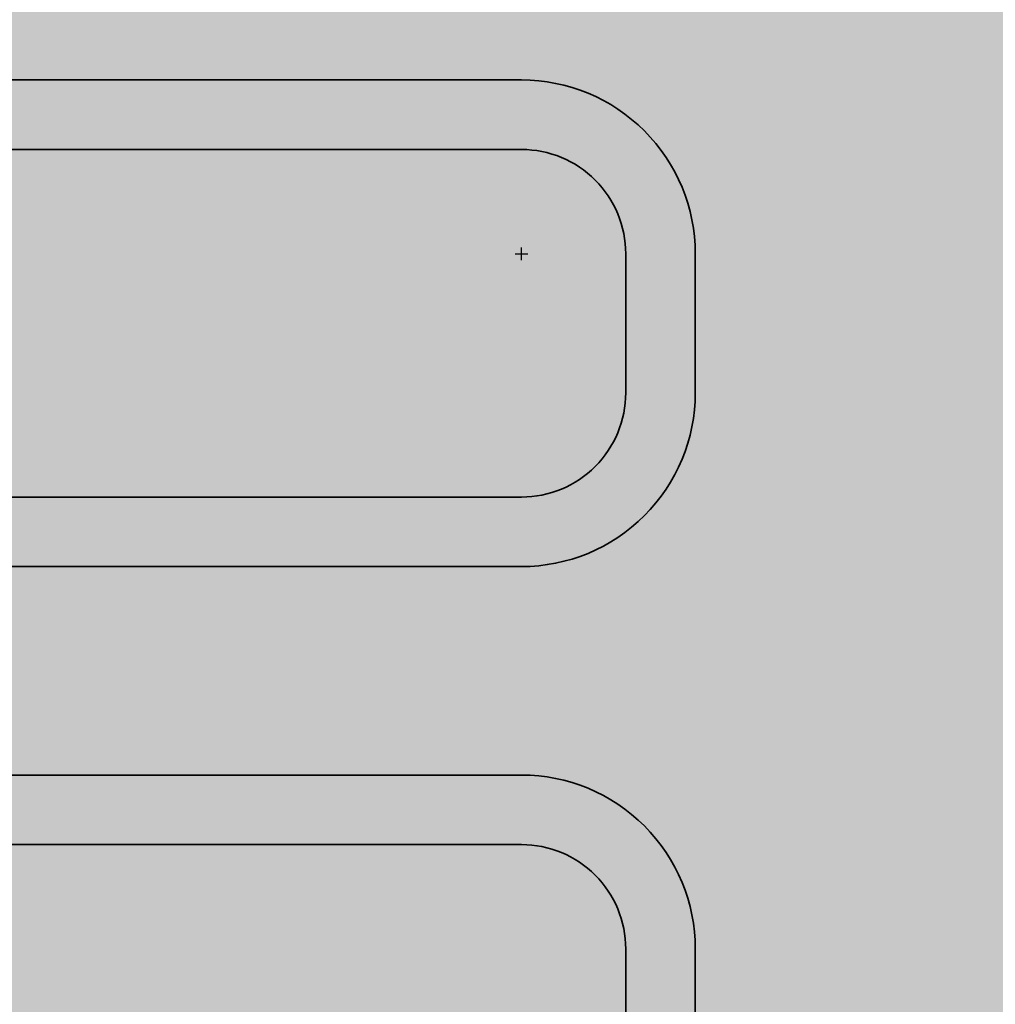
# Model space of a CAD drawing. Units: millimetres. Extents: x -22994 to 29398, y -19990 to 20176.
# Tile 49 of 135: x 169.59 to 183.63, y 110.33 to 124.5. Entities that reach past the tile are written whole.
import ezdxf

# ---------------------------------------------------------------- set-up
doc = ezdxf.new("R2010")
doc.units = ezdxf.units.MM
doc.header["$MEASUREMENT"] = 0
for name, color, linetype, lineweight in [('M-DIMS', 2, 'Continuous', 18), ('M-EQPM-PATT', 7, 'Continuous', 18), ('M-PIPE', 7, 'Continuous', 35)]:
    doc.layers.add(name, color=color, linetype=linetype, lineweight=lineweight)
doc.styles.get("Standard").update_dxf_attribs({"font": 'arial.ttf'})
doc.dimstyles.get("Standard").update_dxf_attribs({"dimtxt": 0.18, "dimasz": 10000, "dimexe": 0.18, "dimexo": 0.0625, "dimgap": 0.09, "dimtad": 0, "dimtih": 1, "dimtoh": 1, "dimdec": 0, "dimzin": 0, "dimdsep": 46, "dimtxsty": 'Standard', "dimcen": 0.09, "dimadec": 0, "dimazin": 0, "dimtfac": 1, "dimtdec": 0, "dimtofl": 0, "dimtmove": 0, "dimatfit": 3, "dimfxl": 1, "dimtolj": 1, "dimtzin": 0, "dimlwd": 30, "dimarcsym": 0})

# ---------------------------------------------------------------- blocks, each defined once
blk = doc.blocks.new('*D2')
at = {"layer": 'Defpoints', "color": 0, "transparency": 16777216}
for p in [(6.677, 10.271), (290.852, 10.271), (290.852, -5.079)]:
    blk.add_point(p, dxfattribs=at)
at = {"layer": 'M-DIMS', "color": 0, "lineweight": -2, "transparency": 16777216}
for p, q in [((6.677, 10.209), (6.677, -5.259)), ((290.852, 10.209), (290.852, -5.259))]:
    blk.add_line(p, q, dxfattribs=at)
at = {"layer": 'M-DIMS', "color": 0, "lineweight": 30, "transparency": 16777216}
for p, q in [((-9993.323, -5.079), (-19993.323, -5.079)), ((10290.852, -5.079), (20290.852, -5.079))]:
    blk.add_line(p, q, dxfattribs=at)
at = {"layer": 'M-DIMS', "color": 0, "transparency": 16777216}
for points in [[(-9993.323, 1661.588), (-9993.323, -1671.745), (6.677, -5.079)], [(10290.852, 1661.588), (10290.852, -1671.745), (290.852, -5.079)]]:
    blk.add_solid(points, dxfattribs=at)
at = {"layer": 'M-DIMS', "color": 0, "transparency": 16777216, "insert": (148.765, -5.079), "char_height": 0.18, "attachment_point": 5}
blk.add_mtext('\\A1;284.2', dxfattribs=at)
blk = doc.blocks.new('*D3')
at = {"layer": 'Defpoints', "color": 0, "transparency": 16777216}
for p in [(110.265, 204.165), (110.265, 176.366), (95.833, 127.967)]:
    blk.add_point(p, dxfattribs=at)
at = {"layer": 'M-DIMS', "color": 0, "lineweight": -2, "transparency": 16777216}
for p, q in [((95.833, 128.03), (95.833, 204.345)), ((110.265, 176.429), (110.265, 204.345))]:
    blk.add_line(p, q, dxfattribs=at)
at = {"layer": 'M-DIMS', "color": 0, "lineweight": 30, "transparency": 16777216}
for p, q in [((-9904.167, 204.165), (-19904.167, 204.165)), ((10110.265, 204.165), (20110.265, 204.165))]:
    blk.add_line(p, q, dxfattribs=at)
at = {"layer": 'M-DIMS', "color": 0, "transparency": 16777216}
for points in [[(-9904.167, 1870.832), (-9904.167, -1462.501), (95.833, 204.165)], [(10110.265, 1870.832), (10110.265, -1462.501), (110.265, 204.165)]]:
    blk.add_solid(points, dxfattribs=at)
at = {"layer": 'M-DIMS', "color": 0, "transparency": 16777216, "insert": (103.049, 204.165), "char_height": 0.18, "attachment_point": 5}
blk.add_mtext('\\A1;14.432', dxfattribs=at)
blk = doc.blocks.new('*D4')
at = {"layer": 'Defpoints', "color": 0, "transparency": 16777216}
for p in [(116.265, 204.165), (110.265, 176.366), (116.265, 176.366)]:
    blk.add_point(p, dxfattribs=at)
at = {"layer": 'M-DIMS', "color": 0, "lineweight": -2, "transparency": 16777216}
for p, q in [((110.265, 176.429), (110.265, 204.345)), ((116.265, 176.429), (116.265, 204.345))]:
    blk.add_line(p, q, dxfattribs=at)
at = {"layer": 'M-DIMS', "color": 0, "lineweight": 30, "transparency": 16777216}
for p, q in [((-9889.735, 204.165), (-19889.735, 204.165)), ((10116.265, 204.165), (20116.265, 204.165))]:
    blk.add_line(p, q, dxfattribs=at)
at = {"layer": 'M-DIMS', "color": 0, "transparency": 16777216}
for points in [[(-9889.735, 1870.832), (-9889.735, -1462.501), (110.265, 204.165)], [(10116.265, 1870.832), (10116.265, -1462.501), (116.265, 204.165)]]:
    blk.add_solid(points, dxfattribs=at)
at = {"layer": 'M-DIMS', "color": 0, "transparency": 16777216, "insert": (113.265, 204.165), "char_height": 0.18, "attachment_point": 5}
blk.add_mtext('\\A1;6', dxfattribs=at)
blk = doc.blocks.new('*D5')
at = {"layer": 'Defpoints', "color": 0, "transparency": 16777216}
for p in [(181.265, 204.165), (116.265, 176.366), (181.265, 176.366)]:
    blk.add_point(p, dxfattribs=at)
at = {"layer": 'M-DIMS', "color": 0, "lineweight": -2, "transparency": 16777216}
for p, q in [((116.265, 176.429), (116.265, 204.345)), ((181.265, 176.429), (181.265, 204.345))]:
    blk.add_line(p, q, dxfattribs=at)
at = {"layer": 'M-DIMS', "color": 0, "lineweight": 30, "transparency": 16777216}
for p, q in [((-9883.735, 204.165), (-19883.735, 204.165)), ((10181.265, 204.165), (20181.265, 204.165))]:
    blk.add_line(p, q, dxfattribs=at)
at = {"layer": 'M-DIMS', "color": 0, "transparency": 16777216}
for points in [[(-9883.735, 1870.832), (-9883.735, -1462.501), (116.265, 204.165)], [(10181.265, 1870.832), (10181.265, -1462.501), (181.265, 204.165)]]:
    blk.add_solid(points, dxfattribs=at)
at = {"layer": 'M-DIMS', "color": 0, "transparency": 16777216, "insert": (148.765, 204.165), "char_height": 0.18, "attachment_point": 5}
blk.add_mtext('\\A1;65', dxfattribs=at)
blk = doc.blocks.new('*D6')
at = {"layer": 'Defpoints', "color": 0, "transparency": 16777216}
for p in [(187.265, 204.165), (181.265, 176.366), (187.265, 176.366)]:
    blk.add_point(p, dxfattribs=at)
at = {"layer": 'M-DIMS', "color": 0, "lineweight": -2, "transparency": 16777216}
for p, q in [((181.265, 176.429), (181.265, 204.345)), ((187.265, 176.429), (187.265, 204.345))]:
    blk.add_line(p, q, dxfattribs=at)
at = {"layer": 'M-DIMS', "color": 0, "lineweight": 30, "transparency": 16777216}
for p, q in [((-9818.735, 204.165), (-19818.735, 204.165)), ((10187.265, 204.165), (20187.265, 204.165))]:
    blk.add_line(p, q, dxfattribs=at)
at = {"layer": 'M-DIMS', "color": 0, "transparency": 16777216}
for points in [[(-9818.735, 1870.832), (-9818.735, -1462.501), (181.265, 204.165)], [(10187.265, 1870.832), (10187.265, -1462.501), (187.265, 204.165)]]:
    blk.add_solid(points, dxfattribs=at)
at = {"layer": 'M-DIMS', "color": 0, "transparency": 16777216, "insert": (184.265, 204.165), "char_height": 0.18, "attachment_point": 5}
blk.add_mtext('\\A1;6', dxfattribs=at)
blk = doc.blocks.new('*D7')
at = {"layer": 'Defpoints', "color": 0, "transparency": 16777216}
for p in [(201.697, 204.165), (187.265, 176.366), (201.697, 127.967)]:
    blk.add_point(p, dxfattribs=at)
at = {"layer": 'M-DIMS', "color": 0, "lineweight": -2, "transparency": 16777216}
for p, q in [((187.265, 176.429), (187.265, 204.345)), ((201.697, 128.03), (201.697, 204.345))]:
    blk.add_line(p, q, dxfattribs=at)
at = {"layer": 'M-DIMS', "color": 0, "lineweight": 30, "transparency": 16777216}
for p, q in [((-9812.735, 204.165), (-19812.735, 204.165)), ((10201.697, 204.165), (20201.697, 204.165))]:
    blk.add_line(p, q, dxfattribs=at)
at = {"layer": 'M-DIMS', "color": 0, "transparency": 16777216}
for points in [[(-9812.735, 1870.832), (-9812.735, -1462.501), (187.265, 204.165)], [(10201.697, 1870.832), (10201.697, -1462.501), (201.697, 204.165)]]:
    blk.add_solid(points, dxfattribs=at)
at = {"layer": 'M-DIMS', "color": 0, "transparency": 16777216, "insert": (194.481, 204.165), "char_height": 0.18, "attachment_point": 5}
blk.add_mtext('\\A1;14.432', dxfattribs=at)
blk = doc.blocks.new('*D8')
at = {"layer": 'Defpoints', "color": 0, "transparency": 16777216}
for p in [(227.648, 204.165), (227.648, 146.73), (201.697, 127.967)]:
    blk.add_point(p, dxfattribs=at)
at = {"layer": 'M-DIMS', "color": 0, "lineweight": -2, "transparency": 16777216}
for p, q in [((201.697, 128.03), (201.697, 204.345)), ((227.648, 146.792), (227.648, 204.345))]:
    blk.add_line(p, q, dxfattribs=at)
at = {"layer": 'M-DIMS', "color": 0, "lineweight": 30, "transparency": 16777216}
for p, q in [((-9798.303, 204.165), (-19798.303, 204.165)), ((10227.648, 204.165), (20227.648, 204.165))]:
    blk.add_line(p, q, dxfattribs=at)
at = {"layer": 'M-DIMS', "color": 0, "transparency": 16777216}
for points in [[(-9798.303, 1870.832), (-9798.303, -1462.501), (201.697, 204.165)], [(10227.648, 1870.832), (10227.648, -1462.501), (227.648, 204.165)]]:
    blk.add_solid(points, dxfattribs=at)
at = {"layer": 'M-DIMS', "color": 0, "transparency": 16777216, "insert": (214.673, 204.165), "char_height": 0.18, "attachment_point": 5}
blk.add_mtext('\\A1;25.95', dxfattribs=at)
blk = doc.blocks.new('*D9')
at = {"layer": 'Defpoints', "color": 0, "transparency": 16777216}
for p in [(187.265, 176.366), (306.202, 176.366), (290.852, 10.271)]:
    blk.add_point(p, dxfattribs=at)
at = {"layer": 'M-DIMS', "color": 0, "lineweight": 30, "transparency": 16777216}
for p, q in [((306.202, 10176.366), (306.202, 20176.366)), ((306.202, -9989.729), (306.202, -19989.729))]:
    blk.add_line(p, q, dxfattribs=at)
at = {"layer": 'M-DIMS', "color": 0, "lineweight": -2, "transparency": 16777216}
for p, q in [((187.327, 176.366), (306.382, 176.366)), ((290.915, 10.271), (306.382, 10.271))]:
    blk.add_line(p, q, dxfattribs=at)
at = {"layer": 'M-DIMS', "color": 0, "transparency": 16777216}
for points in [[(-1360.465, 10176.366), (1972.869, 10176.366), (306.202, 176.366)], [(-1360.465, -9989.729), (1972.869, -9989.729), (306.202, 10.271)]]:
    blk.add_solid(points, dxfattribs=at)
at = {"layer": 'M-DIMS', "color": 0, "transparency": 16777216, "insert": (306.202, 93.319), "char_height": 0.18, "attachment_point": 5}
blk.add_mtext('\\A1;166.1', dxfattribs=at)
blk = doc.blocks.new('*D10')
at = {"layer": 'Defpoints', "color": 0, "transparency": 16777216}
for p in [(125.65, 136.071), (133.346, 136.071), (133.346, -5.079)]:
    blk.add_point(p, dxfattribs=at)
at = {"layer": 'M-DIMS', "color": 0, "lineweight": -2, "transparency": 16777216}
for p, q in [((125.65, 136.009), (125.65, -5.259)), ((133.346, 136.009), (133.346, -5.259))]:
    blk.add_line(p, q, dxfattribs=at)
at = {"layer": 'M-DIMS', "color": 0, "lineweight": 30, "transparency": 16777216}
for p, q in [((-9874.35, -5.079), (-19874.35, -5.079)), ((10133.346, -5.079), (20133.346, -5.079))]:
    blk.add_line(p, q, dxfattribs=at)
at = {"layer": 'M-DIMS', "color": 0, "transparency": 16777216}
for points in [[(-9874.35, 1661.588), (-9874.35, -1671.745), (125.65, -5.079)], [(10133.346, 1661.588), (10133.346, -1671.745), (133.346, -5.079)]]:
    blk.add_solid(points, dxfattribs=at)
at = {"layer": 'M-DIMS', "color": 0, "transparency": 16777216, "insert": (129.498, -5.079), "char_height": 0.18, "attachment_point": 5}
blk.add_mtext('\\A1;7.696', dxfattribs=at)
blk = doc.blocks.new('*D11')
at = {"layer": 'Defpoints', "color": 0, "transparency": 16777216}
for p in [(133.346, 136.071), (135.65, 136.071), (135.65, -5.079)]:
    blk.add_point(p, dxfattribs=at)
at = {"layer": 'M-DIMS', "color": 0, "lineweight": -2, "transparency": 16777216}
for p, q in [((133.346, 136.009), (133.346, -5.259)), ((135.65, 136.009), (135.65, -5.259))]:
    blk.add_line(p, q, dxfattribs=at)
at = {"layer": 'M-DIMS', "color": 0, "lineweight": 30, "transparency": 16777216}
for p, q in [((-9866.654, -5.079), (-19866.654, -5.079)), ((10135.65, -5.079), (20135.65, -5.079))]:
    blk.add_line(p, q, dxfattribs=at)
at = {"layer": 'M-DIMS', "color": 0, "transparency": 16777216}
for points in [[(-9866.654, 1661.588), (-9866.654, -1671.745), (133.346, -5.079)], [(10135.65, 1661.588), (10135.65, -1671.745), (135.65, -5.079)]]:
    blk.add_solid(points, dxfattribs=at)
at = {"layer": 'M-DIMS', "color": 0, "transparency": 16777216, "insert": (134.498, -5.079), "char_height": 0.18, "attachment_point": 5}
blk.add_mtext('\\A1;2.304', dxfattribs=at)
blk = doc.blocks.new('*D12')
at = {"layer": 'Defpoints', "color": 0, "transparency": 16777216}
for p in [(135.65, 136.071), (145.65, 136.071), (145.65, -5.079)]:
    blk.add_point(p, dxfattribs=at)
at = {"layer": 'M-DIMS', "color": 0, "lineweight": -2, "transparency": 16777216}
for p, q in [((135.65, 136.009), (135.65, -5.259)), ((145.65, 136.009), (145.65, -5.259))]:
    blk.add_line(p, q, dxfattribs=at)
at = {"layer": 'M-DIMS', "color": 0, "lineweight": 30, "transparency": 16777216}
for p, q in [((-9864.35, -5.079), (-19864.35, -5.079)), ((10145.65, -5.079), (20145.65, -5.079))]:
    blk.add_line(p, q, dxfattribs=at)
at = {"layer": 'M-DIMS', "color": 0, "transparency": 16777216}
for points in [[(-9864.35, 1661.588), (-9864.35, -1671.745), (135.65, -5.079)], [(10145.65, 1661.588), (10145.65, -1671.745), (145.65, -5.079)]]:
    blk.add_solid(points, dxfattribs=at)
at = {"layer": 'M-DIMS', "color": 0, "transparency": 16777216, "insert": (140.65, -5.079), "char_height": 0.18, "attachment_point": 5}
blk.add_mtext('\\A1;10', dxfattribs=at)
blk = doc.blocks.new('*D13')
at = {"layer": 'Defpoints', "color": 0, "transparency": 16777216}
for p in [(145.65, 136.071), (155.65, 136.071), (155.65, -5.079)]:
    blk.add_point(p, dxfattribs=at)
at = {"layer": 'M-DIMS', "color": 0, "lineweight": -2, "transparency": 16777216}
for p, q in [((145.65, 136.009), (145.65, -5.259)), ((155.65, 136.009), (155.65, -5.259))]:
    blk.add_line(p, q, dxfattribs=at)
at = {"layer": 'M-DIMS', "color": 0, "lineweight": 30, "transparency": 16777216}
for p, q in [((-9854.35, -5.079), (-19854.35, -5.079)), ((10155.65, -5.079), (20155.65, -5.079))]:
    blk.add_line(p, q, dxfattribs=at)
at = {"layer": 'M-DIMS', "color": 0, "transparency": 16777216}
for points in [[(-9854.35, 1661.588), (-9854.35, -1671.745), (145.65, -5.079)], [(10155.65, 1661.588), (10155.65, -1671.745), (155.65, -5.079)]]:
    blk.add_solid(points, dxfattribs=at)
at = {"layer": 'M-DIMS', "color": 0, "transparency": 16777216, "insert": (150.65, -5.079), "char_height": 0.18, "attachment_point": 5}
blk.add_mtext('\\A1;10', dxfattribs=at)
blk = doc.blocks.new('*D14')
at = {"layer": 'Defpoints', "color": 0, "transparency": 16777216}
for p in [(155.65, 136.071), (165.65, 136.071), (165.65, -5.079)]:
    blk.add_point(p, dxfattribs=at)
at = {"layer": 'M-DIMS', "color": 0, "lineweight": -2, "transparency": 16777216}
for p, q in [((155.65, 136.009), (155.65, -5.259)), ((165.65, 136.009), (165.65, -5.259))]:
    blk.add_line(p, q, dxfattribs=at)
at = {"layer": 'M-DIMS', "color": 0, "lineweight": 30, "transparency": 16777216}
for p, q in [((-9844.35, -5.079), (-19844.35, -5.079)), ((10165.65, -5.079), (20165.65, -5.079))]:
    blk.add_line(p, q, dxfattribs=at)
at = {"layer": 'M-DIMS', "color": 0, "transparency": 16777216}
for points in [[(-9844.35, 1661.588), (-9844.35, -1671.745), (155.65, -5.079)], [(10165.65, 1661.588), (10165.65, -1671.745), (165.65, -5.079)]]:
    blk.add_solid(points, dxfattribs=at)
at = {"layer": 'M-DIMS', "color": 0, "transparency": 16777216, "insert": (160.65, -5.079), "char_height": 0.18, "attachment_point": 5}
blk.add_mtext('\\A1;10', dxfattribs=at)
blk = doc.blocks.new('*D15')
at = {"layer": 'Defpoints', "color": 0, "transparency": 16777216}
for p in [(173.346, 154.788), (173.346, 136.071), (306.202, 136.071)]:
    blk.add_point(p, dxfattribs=at)
at = {"layer": 'M-DIMS', "color": 0, "lineweight": 30, "transparency": 16777216}
for p, q in [((306.202, 10154.788), (306.202, 20154.788)), ((306.202, -9863.929), (306.202, -19863.929))]:
    blk.add_line(p, q, dxfattribs=at)
at = {"layer": 'M-DIMS', "color": 0, "lineweight": -2, "transparency": 16777216}
for p, q in [((173.408, 154.788), (306.382, 154.788)), ((173.408, 136.071), (306.382, 136.071))]:
    blk.add_line(p, q, dxfattribs=at)
at = {"layer": 'M-DIMS', "color": 0, "transparency": 16777216}
for points in [[(-1360.465, 10154.788), (1972.869, 10154.788), (306.202, 154.788)], [(-1360.465, -9863.929), (1972.869, -9863.929), (306.202, 136.071)]]:
    blk.add_solid(points, dxfattribs=at)
at = {"layer": 'M-DIMS', "color": 0, "transparency": 16777216, "insert": (306.202, 145.43), "char_height": 0.18, "attachment_point": 5}
blk.add_mtext('\\A1;18.717', dxfattribs=at)
blk = doc.blocks.new('*D16')
at = {"layer": 'Defpoints', "color": 0, "transparency": 16777216}
for p in [(120.17, 204.165), (110.466, 48.035), (120.17, 48.035)]:
    blk.add_point(p, dxfattribs=at)
at = {"layer": 'M-DIMS', "color": 0, "lineweight": -2, "transparency": 16777216}
for p, q in [((110.466, 48.097), (110.466, 204.345)), ((120.17, 48.097), (120.17, 204.345))]:
    blk.add_line(p, q, dxfattribs=at)
at = {"layer": 'M-DIMS', "color": 0, "lineweight": 30, "transparency": 16777216}
for p, q in [((-9889.534, 204.165), (-19889.534, 204.165)), ((10120.17, 204.165), (20120.17, 204.165))]:
    blk.add_line(p, q, dxfattribs=at)
at = {"layer": 'M-DIMS', "color": 0, "transparency": 16777216}
for points in [[(-9889.534, 1870.832), (-9889.534, -1462.501), (110.466, 204.165)], [(10120.17, 1870.832), (10120.17, -1462.501), (120.17, 204.165)]]:
    blk.add_solid(points, dxfattribs=at)
at = {"layer": 'M-DIMS', "color": 0, "transparency": 16777216, "insert": (115.318, 204.165), "char_height": 0.18, "attachment_point": 5}
blk.add_mtext('\\A1;9.704', dxfattribs=at)
blk = doc.blocks.new('*D17')
at = {"layer": 'Defpoints', "color": 0, "transparency": 16777216}
for p in [(126.17, 204.165), (120.17, 48.035), (126.17, 48.035)]:
    blk.add_point(p, dxfattribs=at)
at = {"layer": 'M-DIMS', "color": 0, "lineweight": -2, "transparency": 16777216}
for p, q in [((120.17, 48.097), (120.17, 204.345)), ((126.17, 48.097), (126.17, 204.345))]:
    blk.add_line(p, q, dxfattribs=at)
at = {"layer": 'M-DIMS', "color": 0, "lineweight": 30, "transparency": 16777216}
for p, q in [((-9879.83, 204.165), (-19879.83, 204.165)), ((10126.17, 204.165), (20126.17, 204.165))]:
    blk.add_line(p, q, dxfattribs=at)
at = {"layer": 'M-DIMS', "color": 0, "transparency": 16777216}
for points in [[(-9879.83, 1870.832), (-9879.83, -1462.501), (120.17, 204.165)], [(10126.17, 1870.832), (10126.17, -1462.501), (126.17, 204.165)]]:
    blk.add_solid(points, dxfattribs=at)
at = {"layer": 'M-DIMS', "color": 0, "transparency": 16777216, "insert": (123.17, 204.165), "char_height": 0.18, "attachment_point": 5}
blk.add_mtext('\\A1;6', dxfattribs=at)
blk = doc.blocks.new('*D18')
at = {"layer": 'Defpoints', "color": 0, "transparency": 16777216}
for p in [(132.17, 204.165), (126.17, 48.035), (132.17, 48.035)]:
    blk.add_point(p, dxfattribs=at)
at = {"layer": 'M-DIMS', "color": 0, "lineweight": -2, "transparency": 16777216}
for p, q in [((126.17, 48.097), (126.17, 204.345)), ((132.17, 48.097), (132.17, 204.345))]:
    blk.add_line(p, q, dxfattribs=at)
at = {"layer": 'M-DIMS', "color": 0, "lineweight": 30, "transparency": 16777216}
for p, q in [((-9873.83, 204.165), (-19873.83, 204.165)), ((10132.17, 204.165), (20132.17, 204.165))]:
    blk.add_line(p, q, dxfattribs=at)
at = {"layer": 'M-DIMS', "color": 0, "transparency": 16777216}
for points in [[(-9873.83, 1870.832), (-9873.83, -1462.501), (126.17, 204.165)], [(10132.17, 1870.832), (10132.17, -1462.501), (132.17, 204.165)]]:
    blk.add_solid(points, dxfattribs=at)
at = {"layer": 'M-DIMS', "color": 0, "transparency": 16777216, "insert": (129.17, 204.165), "char_height": 0.18, "attachment_point": 5}
blk.add_mtext('\\A1;6', dxfattribs=at)
blk = doc.blocks.new('*D19')
at = {"layer": 'Defpoints', "color": 0, "transparency": 16777216}
for p in [(138.17, 204.165), (132.17, 48.035), (138.17, 48.035)]:
    blk.add_point(p, dxfattribs=at)
at = {"layer": 'M-DIMS', "color": 0, "lineweight": -2, "transparency": 16777216}
for p, q in [((132.17, 48.097), (132.17, 204.345)), ((138.17, 48.097), (138.17, 204.345))]:
    blk.add_line(p, q, dxfattribs=at)
at = {"layer": 'M-DIMS', "color": 0, "lineweight": 30, "transparency": 16777216}
for p, q in [((-9867.83, 204.165), (-19867.83, 204.165)), ((10138.17, 204.165), (20138.17, 204.165))]:
    blk.add_line(p, q, dxfattribs=at)
at = {"layer": 'M-DIMS', "color": 0, "transparency": 16777216}
for points in [[(-9867.83, 1870.832), (-9867.83, -1462.501), (132.17, 204.165)], [(10138.17, 1870.832), (10138.17, -1462.501), (138.17, 204.165)]]:
    blk.add_solid(points, dxfattribs=at)
at = {"layer": 'M-DIMS', "color": 0, "transparency": 16777216, "insert": (135.17, 204.165), "char_height": 0.18, "attachment_point": 5}
blk.add_mtext('\\A1;6', dxfattribs=at)
blk = doc.blocks.new('*D20')
at = {"layer": 'Defpoints', "color": 0, "transparency": 16777216}
for p in [(144.17, 204.165), (138.17, 48.035), (144.17, 48.035)]:
    blk.add_point(p, dxfattribs=at)
at = {"layer": 'M-DIMS', "color": 0, "lineweight": -2, "transparency": 16777216}
for p, q in [((138.17, 48.097), (138.17, 204.345)), ((144.17, 48.097), (144.17, 204.345))]:
    blk.add_line(p, q, dxfattribs=at)
at = {"layer": 'M-DIMS', "color": 0, "lineweight": 30, "transparency": 16777216}
for p, q in [((-9861.83, 204.165), (-19861.83, 204.165)), ((10144.17, 204.165), (20144.17, 204.165))]:
    blk.add_line(p, q, dxfattribs=at)
at = {"layer": 'M-DIMS', "color": 0, "transparency": 16777216}
for points in [[(-9861.83, 1870.832), (-9861.83, -1462.501), (138.17, 204.165)], [(10144.17, 1870.832), (10144.17, -1462.501), (144.17, 204.165)]]:
    blk.add_solid(points, dxfattribs=at)
at = {"layer": 'M-DIMS', "color": 0, "transparency": 16777216, "insert": (141.17, 204.165), "char_height": 0.18, "attachment_point": 5}
blk.add_mtext('\\A1;6', dxfattribs=at)
blk = doc.blocks.new('*D21')
at = {"layer": 'Defpoints', "color": 0, "transparency": 16777216}
for p in [(149.116, 204.165), (144.17, 48.035), (149.116, 48.035)]:
    blk.add_point(p, dxfattribs=at)
at = {"layer": 'M-DIMS', "color": 0, "lineweight": -2, "transparency": 16777216}
for p, q in [((144.17, 48.097), (144.17, 204.345)), ((149.116, 48.097), (149.116, 204.345))]:
    blk.add_line(p, q, dxfattribs=at)
at = {"layer": 'M-DIMS', "color": 0, "lineweight": 30, "transparency": 16777216}
for p, q in [((-9855.83, 204.165), (-19855.83, 204.165)), ((10149.116, 204.165), (20149.116, 204.165))]:
    blk.add_line(p, q, dxfattribs=at)
at = {"layer": 'M-DIMS', "color": 0, "transparency": 16777216}
for points in [[(-9855.83, 1870.832), (-9855.83, -1462.501), (144.17, 204.165)], [(10149.116, 1870.832), (10149.116, -1462.501), (149.116, 204.165)]]:
    blk.add_solid(points, dxfattribs=at)
at = {"layer": 'M-DIMS', "color": 0, "transparency": 16777216, "insert": (146.643, 204.165), "char_height": 0.18, "attachment_point": 5}
blk.add_mtext('\\A1;4.945', dxfattribs=at)
blk = doc.blocks.new('*D22')
at = {"layer": 'Defpoints', "color": 0, "transparency": 16777216}
for p in [(149.116, 30.99), (155.116, 30.99), (155.116, -5.079)]:
    blk.add_point(p, dxfattribs=at)
at = {"layer": 'M-DIMS', "color": 0, "lineweight": -2, "transparency": 16777216}
for p, q in [((149.116, 30.927), (149.116, -5.259)), ((155.116, 30.927), (155.116, -5.259))]:
    blk.add_line(p, q, dxfattribs=at)
at = {"layer": 'M-DIMS', "color": 0, "lineweight": 30, "transparency": 16777216}
for p, q in [((-9850.884, -5.079), (-19850.884, -5.079)), ((10155.116, -5.079), (20155.116, -5.079))]:
    blk.add_line(p, q, dxfattribs=at)
at = {"layer": 'M-DIMS', "color": 0, "transparency": 16777216}
for points in [[(-9850.884, 1661.588), (-9850.884, -1671.745), (149.116, -5.079)], [(10155.116, 1661.588), (10155.116, -1671.745), (155.116, -5.079)]]:
    blk.add_solid(points, dxfattribs=at)
at = {"layer": 'M-DIMS', "color": 0, "transparency": 16777216, "insert": (152.116, -5.079), "char_height": 0.18, "attachment_point": 5}
blk.add_mtext('\\A1;6', dxfattribs=at)
blk = doc.blocks.new('*D23')
at = {"layer": 'Defpoints', "color": 0, "transparency": 16777216}
for p in [(155.116, 30.99), (161.116, 30.99), (161.116, -5.079)]:
    blk.add_point(p, dxfattribs=at)
at = {"layer": 'M-DIMS', "color": 0, "lineweight": -2, "transparency": 16777216}
for p, q in [((155.116, 30.927), (155.116, -5.259)), ((161.116, 30.927), (161.116, -5.259))]:
    blk.add_line(p, q, dxfattribs=at)
at = {"layer": 'M-DIMS', "color": 0, "lineweight": 30, "transparency": 16777216}
for p, q in [((-9844.884, -5.079), (-19844.884, -5.079)), ((10161.116, -5.079), (20161.116, -5.079))]:
    blk.add_line(p, q, dxfattribs=at)
at = {"layer": 'M-DIMS', "color": 0, "transparency": 16777216}
for points in [[(-9844.884, 1661.588), (-9844.884, -1671.745), (155.116, -5.079)], [(10161.116, 1661.588), (10161.116, -1671.745), (161.116, -5.079)]]:
    blk.add_solid(points, dxfattribs=at)
at = {"layer": 'M-DIMS', "color": 0, "transparency": 16777216, "insert": (158.116, -5.079), "char_height": 0.18, "attachment_point": 5}
blk.add_mtext('\\A1;6', dxfattribs=at)
blk = doc.blocks.new('*D24')
at = {"layer": 'Defpoints', "color": 0, "transparency": 16777216}
for p in [(161.116, 30.99), (166.439, 30.99), (166.439, -5.079)]:
    blk.add_point(p, dxfattribs=at)
at = {"layer": 'M-DIMS', "color": 0, "lineweight": -2, "transparency": 16777216}
for p, q in [((161.116, 30.927), (161.116, -5.259)), ((166.439, 30.927), (166.439, -5.259))]:
    blk.add_line(p, q, dxfattribs=at)
at = {"layer": 'M-DIMS', "color": 0, "lineweight": 30, "transparency": 16777216}
for p, q in [((-9838.884, -5.079), (-19838.884, -5.079)), ((10166.439, -5.079), (20166.439, -5.079))]:
    blk.add_line(p, q, dxfattribs=at)
at = {"layer": 'M-DIMS', "color": 0, "transparency": 16777216}
for points in [[(-9838.884, 1661.588), (-9838.884, -1671.745), (161.116, -5.079)], [(10166.439, 1661.588), (10166.439, -1671.745), (166.439, -5.079)]]:
    blk.add_solid(points, dxfattribs=at)
at = {"layer": 'M-DIMS', "color": 0, "transparency": 16777216, "insert": (163.777, -5.079), "char_height": 0.18, "attachment_point": 5}
blk.add_mtext('\\A1;5.323', dxfattribs=at)
blk = doc.blocks.new('*D25')
at = {"layer": 'Defpoints', "color": 0, "transparency": 16777216}
for p in [(166.439, 30.99), (172.439, 30.99), (172.439, -5.079)]:
    blk.add_point(p, dxfattribs=at)
at = {"layer": 'M-DIMS', "color": 0, "lineweight": -2, "transparency": 16777216}
for p, q in [((166.439, 30.927), (166.439, -5.259)), ((172.439, 30.927), (172.439, -5.259))]:
    blk.add_line(p, q, dxfattribs=at)
at = {"layer": 'M-DIMS', "color": 0, "lineweight": 30, "transparency": 16777216}
for p, q in [((-9833.561, -5.079), (-19833.561, -5.079)), ((10172.439, -5.079), (20172.439, -5.079))]:
    blk.add_line(p, q, dxfattribs=at)
at = {"layer": 'M-DIMS', "color": 0, "transparency": 16777216}
for points in [[(-9833.561, 1661.588), (-9833.561, -1671.745), (166.439, -5.079)], [(10172.439, 1661.588), (10172.439, -1671.745), (172.439, -5.079)]]:
    blk.add_solid(points, dxfattribs=at)
at = {"layer": 'M-DIMS', "color": 0, "transparency": 16777216, "insert": (169.439, -5.079), "char_height": 0.18, "attachment_point": 5}
blk.add_mtext('\\A1;6', dxfattribs=at)
blk = doc.blocks.new('*D26')
at = {"layer": 'Defpoints', "color": 0, "transparency": 16777216}
for p in [(172.439, 30.99), (178.439, 30.99), (178.439, -5.079)]:
    blk.add_point(p, dxfattribs=at)
at = {"layer": 'M-DIMS', "color": 0, "lineweight": -2, "transparency": 16777216}
for p, q in [((172.439, 30.927), (172.439, -5.259)), ((178.439, 30.927), (178.439, -5.259))]:
    blk.add_line(p, q, dxfattribs=at)
at = {"layer": 'M-DIMS', "color": 0, "lineweight": 30, "transparency": 16777216}
for p, q in [((-9827.561, -5.079), (-19827.561, -5.079)), ((10178.439, -5.079), (20178.439, -5.079))]:
    blk.add_line(p, q, dxfattribs=at)
at = {"layer": 'M-DIMS', "color": 0, "transparency": 16777216}
for points in [[(-9827.561, 1661.588), (-9827.561, -1671.745), (172.439, -5.079)], [(10178.439, 1661.588), (10178.439, -1671.745), (178.439, -5.079)]]:
    blk.add_solid(points, dxfattribs=at)
at = {"layer": 'M-DIMS', "color": 0, "transparency": 16777216, "insert": (175.439, -5.079), "char_height": 0.18, "attachment_point": 5}
blk.add_mtext('\\A1;6', dxfattribs=at)
blk = doc.blocks.new('*D27')
at = {"layer": 'Defpoints', "color": 0, "transparency": 16777216}
for p in [(178.439, 30.99), (188.117, 30.99), (188.117, -5.079)]:
    blk.add_point(p, dxfattribs=at)
at = {"layer": 'M-DIMS', "color": 0, "lineweight": -2, "transparency": 16777216}
for p, q in [((178.439, 30.927), (178.439, -5.259)), ((188.117, 30.927), (188.117, -5.259))]:
    blk.add_line(p, q, dxfattribs=at)
at = {"layer": 'M-DIMS', "color": 0, "lineweight": 30, "transparency": 16777216}
for p, q in [((-9821.561, -5.079), (-19821.561, -5.079)), ((10188.117, -5.079), (20188.117, -5.079))]:
    blk.add_line(p, q, dxfattribs=at)
at = {"layer": 'M-DIMS', "color": 0, "transparency": 16777216}
for points in [[(-9821.561, 1661.588), (-9821.561, -1671.745), (178.439, -5.079)], [(10188.117, 1661.588), (10188.117, -1671.745), (188.117, -5.079)]]:
    blk.add_solid(points, dxfattribs=at)
at = {"layer": 'M-DIMS', "color": 0, "transparency": 16777216, "insert": (183.278, -5.079), "char_height": 0.18, "attachment_point": 5}
blk.add_mtext('\\A1;9.679', dxfattribs=at)
blk = doc.blocks.new('*D28')
at = {"layer": 'Defpoints', "color": 0, "transparency": 16777216}
for p in [(188.117, 48.035), (306.202, 48.035), (188.117, 30.99)]:
    blk.add_point(p, dxfattribs=at)
at = {"layer": 'M-DIMS', "color": 0, "lineweight": 30, "transparency": 16777216}
for p, q in [((306.202, 10048.035), (306.202, 20048.035)), ((306.202, -9969.01), (306.202, -19969.01))]:
    blk.add_line(p, q, dxfattribs=at)
at = {"layer": 'M-DIMS', "color": 0, "lineweight": -2, "transparency": 16777216}
for p, q in [((188.18, 48.035), (306.382, 48.035)), ((188.18, 30.99), (306.382, 30.99))]:
    blk.add_line(p, q, dxfattribs=at)
at = {"layer": 'M-DIMS', "color": 0, "transparency": 16777216}
for points in [[(-1360.465, 10048.035), (1972.869, 10048.035), (306.202, 48.035)], [(-1360.465, -9969.01), (1972.869, -9969.01), (306.202, 30.99)]]:
    blk.add_solid(points, dxfattribs=at)
at = {"layer": 'M-DIMS', "color": 0, "transparency": 16777216, "insert": (306.202, 39.512), "char_height": 0.18, "attachment_point": 5}
blk.add_mtext('\\A1;17.045', dxfattribs=at)
blk = doc.blocks.new('*D29')
at = {"layer": 'Defpoints', "color": 0, "transparency": 16777216}
for p in [(36.801, 80.045), (64.03, 80.045)]:
    blk.add_point(p, dxfattribs=at)
at = {"layer": 'M-DIMS', "color": 0, "lineweight": -2, "transparency": 16777216}
for p, q in [((50.325, 80.045), (50.505, 80.045)), ((50.415, 79.955), (50.415, 80.135))]:
    blk.add_line(p, q, dxfattribs=at)
at = {"layer": 'M-DIMS', "color": 0, "lineweight": 30, "transparency": 16777216}
blk.add_line((20064.03, 80.03), (10064.03, 80.038), dxfattribs=at)
at = {"layer": 'M-DIMS', "color": 0, "transparency": 16777216}
blk.add_solid([(10064.031, 1746.704), (10064.028, -1586.629), (64.03, 80.045)], dxfattribs=at)
at = {"layer": 'M-DIMS', "color": 0, "transparency": 16777216, "insert": (20064.521, 80.03), "char_height": 0.18, "attachment_point": 5}
blk.add_mtext('\\A1;∅27.23', dxfattribs=at)
blk = doc.blocks.new('*D34')
at = {"layer": 'Defpoints', "color": 0, "transparency": 16777216}
for p in [(178.58, 122.895), (176.812, 121.128)]:
    blk.add_point(p, dxfattribs=at)
at = {"layer": 'M-DIMS', "color": 0, "lineweight": 30, "transparency": 16777216}
for p, q in [((14322.436, 14263.311), (7250.508, 7193.103)), ((24322.436, 14263.311), (14322.436, 14263.311))]:
    blk.add_line(p, q, dxfattribs=at)
at = {"layer": 'M-DIMS', "color": 0, "lineweight": -2, "transparency": 16777216}
for p, q in [((176.722, 121.128), (176.902, 121.128)), ((176.812, 121.038), (176.812, 121.218))]:
    blk.add_line(p, q, dxfattribs=at)
at = {"layer": 'M-DIMS', "color": 0, "transparency": 16777216}
blk.add_solid([(6072.14, 8371.758), (8428.876, 6014.448), (178.58, 122.895)], dxfattribs=at)
at = {"layer": 'M-DIMS', "color": 0, "transparency": 16777216, "insert": (24322.97, 14263.311), "char_height": 0.18, "attachment_point": 5}
blk.add_mtext('\\A1;6X R2.5', dxfattribs=at)
blk = doc.blocks.new('*D36')
at = {"layer": 'Defpoints', "color": 0, "transparency": 16777216}
for p in [(46.39, 31.303), (46.387, 26.593)]:
    blk.add_point(p, dxfattribs=at)
at = {"layer": 'M-DIMS', "color": 0, "lineweight": 30, "transparency": 16777216}
for p, q in [((57.15, 20031.301), (51.77, 10031.302)), ((10057.15, 20031.301), (57.15, 20031.301))]:
    blk.add_line(p, q, dxfattribs=at)
at = {"layer": 'M-DIMS', "color": 0, "lineweight": -2, "transparency": 16777216}
for p, q in [((46.299, 28.948), (46.479, 28.948)), ((46.389, 28.858), (46.389, 29.038))]:
    blk.add_line(p, q, dxfattribs=at)
at = {"layer": 'M-DIMS', "color": 0, "transparency": 16777216}
blk.add_solid([(-1614.896, 10032.199), (1718.436, 10030.405), (46.39, 31.303)], dxfattribs=at)
at = {"layer": 'M-DIMS', "color": 0, "transparency": 16777216, "insert": (10057.554, 20031.301), "char_height": 0.18, "attachment_point": 5}
blk.add_mtext('\\A1;∅4.71', dxfattribs=at)
blk = doc.blocks.new('*D37')
at = {"layer": 'Defpoints', "color": 0, "transparency": 16777216}
for p in [(54.834, 118.615), (59.494, 118.614)]:
    blk.add_point(p, dxfattribs=at)
at = {"layer": 'M-DIMS', "color": 0, "lineweight": -2, "transparency": 16777216}
for p, q in [((57.074, 118.614), (57.254, 118.614)), ((57.164, 118.524), (57.164, 118.704))]:
    blk.add_line(p, q, dxfattribs=at)
at = {"layer": 'M-DIMS', "color": 0, "lineweight": 30, "transparency": 16777216}
blk.add_line((20059.493, 116.253), (10059.494, 117.434), dxfattribs=at)
at = {"layer": 'M-DIMS', "color": 0, "transparency": 16777216}
blk.add_solid([(10059.69, 1784.1), (10059.297, -1549.233), (59.494, 118.614)], dxfattribs=at)
at = {"layer": 'M-DIMS', "color": 0, "transparency": 16777216, "insert": (20059.985, 116.253), "char_height": 0.18, "attachment_point": 5}
blk.add_mtext('\\A1;∅4.659', dxfattribs=at)

msp = doc.modelspace()

# ---------------------------------------------------------------- hatches: boundary and pattern name
at = {"layer": 'M-EQPM-PATT'}
h = msp.add_hatch(color=256, dxfattribs=at)
h.set_gradient(color1=(34, 52, 110), color2=(41, 49, 137), tint=1, name='CYLINDER')
h.paths.add_polyline_path([(101.8327, 123.6277), (101.8327, 122.6277), (176.8123, 122.6277, -0.4142136), (178.3123, 121.1277), (178.3123, 119.1277, -0.4142136), (176.8123, 117.6277), (129.8123, 117.6277, 0.4142136), (128.3123, 116.1277), (128.3123, 114.1277, 0.4142136), (129.8123, 112.6277), (176.8123, 112.6277, -0.4142136), (178.3123, 111.1277), (178.3123, 109.1277, -0.4142136), (176.8123, 107.6277), (129.8123, 107.6277, 0.4142136), (128.3123, 106.1277), (128.3123, 104.1277, 0.4142136), (129.8123, 102.6277), (176.8123, 102.6277, -0.4142136), (178.3123, 101.1277), (178.3123, 99.1277, -0.4142136), (176.8123, 97.6277), (101.8327, 97.6277), (101.8327, 96.6277), (176.8123, 96.6277, 0.4142136), (179.3123, 99.1277), (179.3123, 101.1277, 0.4142136), (176.8123, 103.6277), (129.8123, 103.6277, -0.4142136), (129.3123, 104.1277), (129.3123, 106.1277, -0.4142136), (129.8123, 106.6277), (176.8123, 106.6277, 0.4142136), (179.3123, 109.1277), (179.3123, 111.1277, 0.4142136), (176.8123, 113.6277), (129.8123, 113.6277, -0.4142136), (129.3123, 114.1277), (129.3123, 116.1277, -0.4142136), (129.8123, 116.6277), (176.8123, 116.6277, 0.4142136), (179.3123, 119.1277), (179.3123, 121.1277, 0.4142136), (176.8123, 123.6277)])
h.paths.add_polyline_path([(75.6657, 123.6277), (75.6657, 122.6277), (95.8327, 122.6277), (95.8327, 123.6277)])
h.paths.add_polyline_path([(51.0853, 122.6277, -0.0439182), (51.8797, 123.6277), (38.9157, 123.6277), (38.9157, 122.6277)])
h.paths.add_polyline_path([(95.8327, 96.6277), (95.8327, 97.6277), (22.2694, 97.6277, 0.4142136), (20.7694, 96.1277), (20.7694, 89.8712, 0.4142136), (22.2694, 88.3712), (39.6435, 88.3712, -0.024152), (40.4967, 89.3712), (23.2694, 89.3712, -0.4142136), (21.7694, 90.8712), (21.7694, 95.1277, -0.4142136), (23.2694, 96.6277)])
h.paths.add_polyline_path([(137.7248, 106.4435), (168.6853, 106.4435), (168.6853, 114.6864), (137.7248, 114.6864)], flags=25)

# ---------------------------------------------------------------- linework, layer by layer
at = {"layer": 'M-PIPE'}
for points in [[(101.8327, 123.6277), (176.8123, 123.6277, -0.4142136), (179.3123, 121.1277), (179.3123, 119.1277, -0.4142136), (176.8123, 116.6277), (129.8123, 116.6277, 0.4142136), (129.3123, 116.1277), (129.3123, 114.1277, 0.4142136), (129.8123, 113.6277), (176.8123, 113.6277, -0.4142136), (179.3123, 111.1277), (179.3123, 109.1277, -0.4142136), (176.8123, 106.6277), (129.8123, 106.6277, 0.4142136), (129.3123, 106.1277), (129.3123, 104.1277, 0.4142136), (129.8123, 103.6277), (176.8123, 103.6277, -0.4142136), (179.3123, 101.1277), (179.3123, 99.1277, -0.4142136), (176.8123, 96.6277), (101.8327, 96.6277)], [(101.8327, 122.6277), (176.8123, 122.6277, -0.4142136), (178.3123, 121.1277), (178.3123, 119.1277, -0.4142136), (176.8123, 117.6277), (129.8123, 117.6277, 0.4142136), (128.3123, 116.1277), (128.3123, 114.1277, 0.4142136), (129.8123, 112.6277), (176.8123, 112.6277, -0.4142136), (178.3123, 111.1277), (178.3123, 109.1277, -0.4142136), (176.8123, 107.6277), (129.8123, 107.6277, 0.4142136), (128.3123, 106.1277), (128.3123, 104.1277, 0.4142136), (129.8123, 102.6277), (176.8123, 102.6277, -0.4142136), (178.3123, 101.1277), (178.3123, 99.1277, -0.4142136), (176.8123, 97.6277), (101.8327, 97.6277)]]:
    msp.add_lwpolyline(points, format="xyb", dxfattribs=at)

# ---------------------------------------------------------------- dimensions: what is measured, and where the dimension line sits
at = {"layer": 'M-DIMS'}
for base, p1, p2, override, picture, middle in [((306.202, 176.3662), (290.852, 10.2713), (187.2647, 176.3662), {"dimdec": 1, "dimlfac": 1, "dimrnd": 0, "dimzin": 0, "dimdsep": 46, "dimlunit": 2}, '*D9', (306.202, 93.3187)), ((306.202, 136.0713), (173.3459, 154.788), (173.3459, 136.0713), {"dimdec": 3, "dimlfac": 1, "dimrnd": 0, "dimzin": 0, "dimdsep": 46, "dimlunit": 2}, '*D15', (306.202, 145.4297)), ((306.202, 48.0349), (188.1175, 30.9895), (188.1175, 48.0349), {"dimdec": 3, "dimlfac": 1, "dimrnd": 0, "dimzin": 0, "dimdsep": 46, "dimlunit": 2}, '*D28', (306.202, 39.5122))]:
    dim = msp.add_linear_dim(base=base, p1=p1, p2=p2, angle=90, dimstyle='Standard', override=override, dxfattribs=at)
    dim.commit()
    dim.dimension.update_dxf_attribs({"geometry": picture, "text_midpoint": middle})
dim = msp.add_diameter_dim_2p(p1=(46.3875, 26.5934), p2=(46.39, 31.3035), dimstyle='Standard', override={"dimdec": 2, "dimlfac": 1, "dimrnd": 0, "dimzin": 0, "dimdsep": 46, "dimlunit": 2}, dxfattribs=at)
dim.commit()
dim.dimension.update_dxf_attribs({"geometry": '*D36', "text_midpoint": (10057.5542, 20031.3006), "dimtype": 163})
dim = msp.add_radius_dim(center=(176.8123, 121.1277), mpoint=(178.5802, 122.8952), text='6X <>', dimstyle='Standard', override={"dimdec": 1, "dimlfac": 1, "dimrnd": 0, "dimzin": 0, "dimdsep": 46, "dimlunit": 2}, dxfattribs=at)
dim.commit()
dim.dimension.update_dxf_attribs({"geometry": '*D34', "text_midpoint": (24322.9703, 14263.3108)})
for base, p1, p2, override, picture, middle in [((110.2647, 204.1654), (95.8327, 127.967), (110.2647, 176.3662), {"dimdec": 3, "dimlfac": 1, "dimrnd": 0, "dimzin": 0, "dimdsep": 46, "dimlunit": 2}, '*D3', (103.0487, 204.1654)), ((116.2647, 204.1654), (110.2647, 176.3662), (116.2647, 176.3662), {"dimdec": 0, "dimlfac": 1, "dimrnd": 0, "dimzin": 0, "dimdsep": 46, "dimlunit": 2}, '*D4', (113.2647, 204.1654)), ((120.1702, 204.1654), (110.4658, 48.0349), (120.1702, 48.0349), {"dimdec": 3, "dimlfac": 1, "dimrnd": 0, "dimzin": 0, "dimdsep": 46, "dimlunit": 2}, '*D16', (115.318, 204.1654)), ((181.2647, 204.1654), (116.2647, 176.3662), (181.2647, 176.3662), {"dimdec": 0, "dimlfac": 1, "dimrnd": 0, "dimzin": 0, "dimdsep": 46, "dimlunit": 2}, '*D5', (148.7647, 204.1654)), ((126.1702, 204.1654), (120.1702, 48.0349), (126.1702, 48.0349), {"dimdec": 0, "dimlfac": 1, "dimrnd": 0, "dimzin": 0, "dimdsep": 46, "dimlunit": 2}, '*D17', (123.1702, 204.1654)), ((132.1702, 204.1654), (126.1702, 48.0349), (132.1702, 48.0349), {"dimdec": 0, "dimlfac": 1, "dimrnd": 0, "dimzin": 0, "dimdsep": 46, "dimlunit": 2}, '*D18', (129.1702, 204.1654)), ((138.1702, 204.1654), (132.1702, 48.0349), (138.1702, 48.0349), {"dimdec": 0, "dimlfac": 1, "dimrnd": 0, "dimzin": 0, "dimdsep": 46, "dimlunit": 2}, '*D19', (135.1702, 204.1654)), ((144.1702, 204.1654), (138.1702, 48.0349), (144.1702, 48.0349), {"dimdec": 0, "dimlfac": 1, "dimrnd": 0, "dimzin": 0, "dimdsep": 46, "dimlunit": 2}, '*D20', (141.1702, 204.1654)), ((149.11567, 204.16539), (144.17023, 48.03494), (149.11567, 48.03494), {"dimdec": 3, "dimlfac": 1, "dimrnd": 0, "dimzin": 0, "dimdsep": 46, "dimlunit": 2}, '*D21', (146.64295, 204.16539)), ((187.2647, 204.1654), (181.2647, 176.3662), (187.2647, 176.3662), {"dimdec": 0, "dimlfac": 1, "dimrnd": 0, "dimzin": 0, "dimdsep": 46, "dimlunit": 2}, '*D6', (184.2647, 204.1654)), ((201.6967, 204.1654), (187.2647, 176.3662), (201.6967, 127.967), {"dimdec": 3, "dimlfac": 1, "dimrnd": 0, "dimzin": 0, "dimdsep": 46, "dimlunit": 2}, '*D7', (194.4807, 204.1654)), ((227.6485, 204.1654), (201.6967, 127.967), (227.6485, 146.7296), {"dimdec": 2, "dimlfac": 1, "dimrnd": 0, "dimzin": 0, "dimdsep": 46, "dimlunit": 2}, '*D8', (214.6726, 204.1654)), ((290.852, -5.0787), (6.6773, 10.2713), (290.852, 10.2713), {"dimdec": 1, "dimlfac": 1, "dimrnd": 0, "dimzin": 0, "dimdsep": 46, "dimlunit": 2}, '*D2', (148.7647, -5.0787)), ((133.3459, -5.0787), (125.6498, 136.0713), (133.3459, 136.0713), {"dimdec": 3, "dimlfac": 1, "dimrnd": 0, "dimzin": 0, "dimdsep": 46, "dimlunit": 2}, '*D10', (129.4978, -5.0787)), ((135.6498, -5.0787), (133.3459, 136.0713), (135.6498, 136.0713), {"dimdec": 3, "dimlfac": 1, "dimrnd": 0, "dimzin": 0, "dimdsep": 46, "dimlunit": 2}, '*D11', (134.4978, -5.0787)), ((145.6498, -5.0787), (135.6498, 136.0713), (145.6498, 136.0713), {"dimdec": 0, "dimlfac": 1, "dimrnd": 0, "dimzin": 0, "dimdsep": 46, "dimlunit": 2}, '*D12', (140.6498, -5.0787)), ((155.6498, -5.0787), (145.6498, 136.0713), (155.6498, 136.0713), {"dimdec": 0, "dimlfac": 1, "dimrnd": 0, "dimzin": 0, "dimdsep": 46, "dimlunit": 2}, '*D13', (150.6498, -5.0787)), ((155.1157, -5.0787), (149.1157, 30.9895), (155.1157, 30.9895), {"dimdec": 0, "dimlfac": 1, "dimrnd": 0, "dimzin": 0, "dimdsep": 46, "dimlunit": 2}, '*D22', (152.1157, -5.0787)), ((161.1157, -5.0787), (155.1157, 30.9895), (161.1157, 30.9895), {"dimdec": 0, "dimlfac": 1, "dimrnd": 0, "dimzin": 0, "dimdsep": 46, "dimlunit": 2}, '*D23', (158.1157, -5.0787)), ((165.6498, -5.0787), (155.6498, 136.0713), (165.6498, 136.0713), {"dimdec": 0, "dimlfac": 1, "dimrnd": 0, "dimzin": 0, "dimdsep": 46, "dimlunit": 2}, '*D14', (160.6498, -5.0787)), ((166.4387, -5.0787), (161.1157, 30.9895), (166.4387, 30.9895), {"dimdec": 3, "dimlfac": 1, "dimrnd": 0, "dimzin": 0, "dimdsep": 46, "dimlunit": 2}, '*D24', (163.7772, -5.0787)), ((172.4387, -5.0787), (166.4387, 30.9895), (172.4387, 30.9895), {"dimdec": 0, "dimlfac": 1, "dimrnd": 0, "dimzin": 0, "dimdsep": 46, "dimlunit": 2}, '*D25', (169.4387, -5.0787)), ((178.4387, -5.0787), (172.4387, 30.9895), (178.4387, 30.9895), {"dimdec": 0, "dimlfac": 1, "dimrnd": 0, "dimzin": 0, "dimdsep": 46, "dimlunit": 2}, '*D26', (175.4387, -5.0787)), ((188.1175, -5.0787), (178.4387, 30.9895), (188.1175, 30.9895), {"dimdec": 3, "dimlfac": 1, "dimrnd": 0, "dimzin": 0, "dimdsep": 46, "dimlunit": 2}, '*D27', (183.2781, -5.0787))]:
    dim = msp.add_linear_dim(base=base, p1=p1, p2=p2, dimstyle='Standard', override=override, dxfattribs=at)
    dim.commit()
    dim.dimension.update_dxf_attribs({"geometry": picture, "text_midpoint": middle})
for p1, p2, override, picture, middle in [((54.8343, 118.6145), (59.4936, 118.614), {"dimdec": 3, "dimlfac": 1, "dimrnd": 0, "dimzin": 0, "dimdsep": 46, "dimlunit": 2}, '*D37', (20059.4934, 116.2531)), ((36.8006, 80.045), (64.0296, 80.045), {"dimdec": 2, "dimlfac": 1, "dimrnd": 0, "dimzin": 0, "dimdsep": 46, "dimlunit": 2}, '*D29', (20064.0296, 80.0303))]:
    dim = msp.add_diameter_dim_2p(p1=p1, p2=p2, dimstyle='Standard', override=override, dxfattribs=at)
    dim.commit()
    dim.dimension.update_dxf_attribs({"geometry": picture, "text_midpoint": middle})

doc.saveas('drawing.dxf')
